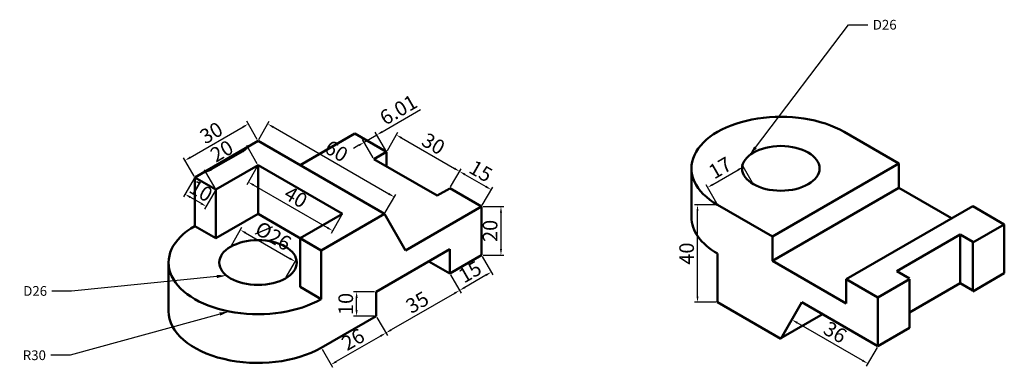
# Model space of a CAD drawing. Units: millimetres. Extents: x 2898 to 3303, y 965 to 1108.
import ezdxf
from ezdxf import colors
from ezdxf.entities.mleader import LeaderData, LeaderLine
from ezdxf.math import Vec2, Vec3

# ---------------------------------------------------------------- set-up
doc = ezdxf.new("R2010")
doc.units = ezdxf.units.MM
doc.layers.add('M-DIMS', color=2, linetype='Continuous', lineweight=25)
doc.layers.add('M-OUTL', color=7, linetype='Continuous', lineweight=50)
doc.styles.get("Standard").update_dxf_attribs({"font": 'arial.ttf'})
doc.dimstyles.new('ISO-25', dxfattribs={"dimtxt": 6, "dimasz": 2.5, "dimexe": 1.25, "dimexo": 0.625, "dimtad": 1, "dimtxsty": 'Standard', "dimcen": 2.5, "dimadec": 0, "dimazin": 0, "dimtfac": 1, "dimtmove": 0, "dimatfit": 3, "dimfxl": 1, "dimarcsym": 0})

# ---------------------------------------------------------------- blocks, each defined once
blk = doc.blocks.new('*D1')
at = {"layer": 'Defpoints', "color": 0, "transparency": 16777216}
for p in [(2992.16, 1065.01), (2996.16, 1058.09), (2970.18, 1043.09)]:
    blk.add_point(p, dxfattribs=at)
at = {"layer": 'M-DIMS', "color": 0, "lineweight": -2, "transparency": 16777216}
for p, q in [((2968.35, 1051.26), (2990, 1063.76)), ((2995.85, 1058.63), (2991.54, 1066.1)), ((2969.87, 1043.63), (2965.56, 1051.1))]:
    blk.add_line(p, q, dxfattribs=at)
at = {"layer": 'M-DIMS', "color": 0, "transparency": 16777216}
for points in [[(2989.79, 1064.12), (2990.21, 1063.4), (2992.16, 1065.01)], [(2968.14, 1051.62), (2968.56, 1050.9), (2966.18, 1050.01)]]:
    blk.add_solid(points, dxfattribs=at)
at = {"layer": 'M-DIMS', "color": 0, "transparency": 16777216, "insert": (2977.33, 1060.71), "char_height": 6, "attachment_point": 5, "rotation": 30}
blk.add_mtext('30', dxfattribs=at)
blk = doc.blocks.new('*D2')
at = {"layer": 'Defpoints', "color": 0, "transparency": 16777216}
for p in [(2992.16, 1055.01), (2996.16, 1048.09), (2978.84, 1038.09)]:
    blk.add_point(p, dxfattribs=at)
at = {"layer": 'M-DIMS', "color": 0, "lineweight": -2, "transparency": 16777216}
for p, q in [((2995.85, 1048.63), (2991.54, 1056.1)), ((2977.01, 1046.26), (2990, 1053.76)), ((2978.53, 1038.63), (2974.22, 1046.1))]:
    blk.add_line(p, q, dxfattribs=at)
at = {"layer": 'M-DIMS', "color": 0, "transparency": 16777216}
for points in [[(2989.79, 1054.12), (2990.21, 1053.4), (2992.16, 1055.01)], [(2976.8, 1046.62), (2977.22, 1045.9), (2974.84, 1045.01)]]:
    blk.add_solid(points, dxfattribs=at)
at = {"layer": 'M-DIMS', "color": 0, "transparency": 16777216, "insert": (2981.66, 1053.21), "char_height": 6, "attachment_point": 5, "rotation": 30}
blk.add_mtext('20', dxfattribs=at)
blk = doc.blocks.new('*D3')
at = {"layer": 'Defpoints', "color": 0, "transparency": 16777216}
for p in [(2996.16, 1048.09), (2992.16, 1041.16), (3030.8, 1028.09)]:
    blk.add_point(p, dxfattribs=at)
at = {"layer": 'M-DIMS', "color": 0, "lineweight": -2, "transparency": 16777216}
for p, q in [((2995.85, 1047.54), (2991.54, 1040.07)), ((3024.64, 1022.41), (2994.33, 1039.91)), ((3030.49, 1027.54), (3026.18, 1020.07))]:
    blk.add_line(p, q, dxfattribs=at)
at = {"layer": 'M-DIMS', "color": 0, "transparency": 16777216}
for points in [[(2994.54, 1040.27), (2994.12, 1039.55), (2992.16, 1041.16)], [(3024.85, 1022.77), (3024.43, 1022.05), (3026.8, 1021.16)]]:
    blk.add_solid(points, dxfattribs=at)
at = {"layer": 'M-DIMS', "color": 0, "transparency": 16777216, "insert": (3011.33, 1034.35), "char_height": 6, "attachment_point": 5, "rotation": 330}
blk.add_mtext('40', dxfattribs=at)
blk = doc.blocks.new('*D4')
at = {"layer": 'Defpoints', "color": 0, "transparency": 16777216}
for p in [(2970.18, 1043.09), (2966.18, 1036.16), (2978.84, 1038.09)]:
    blk.add_point(p, dxfattribs=at)
at = {"layer": 'M-DIMS', "color": 0, "lineweight": -2, "transparency": 16777216}
for p, q in [((2969.87, 1042.54), (2965.56, 1035.07)), ((2978.53, 1037.54), (2974.22, 1030.07)), ((2972.68, 1032.41), (2968.35, 1034.91))]:
    blk.add_line(p, q, dxfattribs=at)
at = {"layer": 'M-DIMS', "color": 0, "transparency": 16777216}
for points in [[(2968.56, 1035.27), (2968.14, 1034.55), (2966.18, 1036.16)], [(2972.89, 1032.77), (2972.47, 1032.05), (2974.84, 1031.16)]]:
    blk.add_solid(points, dxfattribs=at)
at = {"layer": 'M-DIMS', "color": 0, "transparency": 16777216, "insert": (2972.36, 1036.85), "char_height": 6, "attachment_point": 5, "rotation": 330}
blk.add_mtext('10', dxfattribs=at)
blk = doc.blocks.new('*D5')
at = {"layer": 'Defpoints', "color": 0, "transparency": 16777216}
for p in [(3087.96, 1031.09), (3087.96, 1011.09), (3095.96, 1011.09)]:
    blk.add_point(p, dxfattribs=at)
at = {"layer": 'M-DIMS', "color": 0, "lineweight": -2, "transparency": 16777216}
for p, q in [((3088.59, 1031.09), (3097.21, 1031.09)), ((3095.96, 1028.59), (3095.96, 1013.59)), ((3088.59, 1011.09), (3097.21, 1011.09))]:
    blk.add_line(p, q, dxfattribs=at)
at = {"layer": 'M-DIMS', "color": 0, "transparency": 16777216}
for points in [[(3095.55, 1028.59), (3096.38, 1028.59), (3095.96, 1031.09)], [(3095.55, 1013.59), (3096.38, 1013.59), (3095.96, 1011.09)]]:
    blk.add_solid(points, dxfattribs=at)
at = {"layer": 'M-DIMS', "color": 0, "transparency": 16777216, "insert": (3092.27, 1021.09), "char_height": 6, "attachment_point": 5, "rotation": 90}
blk.add_mtext('20', dxfattribs=at)
blk = doc.blocks.new('*D6')
at = {"layer": 'Defpoints', "color": 0, "transparency": 16777216}
for p in [(3044.66, 986.09), (3022.14, 973.09), (3026.14, 966.16)]:
    blk.add_point(p, dxfattribs=at)
at = {"layer": 'M-DIMS', "color": 0, "lineweight": -2, "transparency": 16777216}
for p, q in [((3044.97, 985.54), (3049.29, 978.07)), ((3046.5, 977.91), (3028.31, 967.41)), ((3022.46, 972.54), (3026.77, 965.07))]:
    blk.add_line(p, q, dxfattribs=at)
at = {"layer": 'M-DIMS', "color": 0, "transparency": 16777216}
for points in [[(3046.29, 978.27), (3046.7, 977.55), (3048.66, 979.16)], [(3028.1, 967.77), (3028.52, 967.05), (3026.14, 966.16)]]:
    blk.add_solid(points, dxfattribs=at)
at = {"layer": 'M-DIMS', "color": 0, "transparency": 16777216, "insert": (3035.56, 975.85), "char_height": 6, "attachment_point": 5, "rotation": 30}
blk.add_mtext('26', dxfattribs=at)
blk = doc.blocks.new('*D7')
at = {"layer": 'Defpoints', "color": 0, "transparency": 16777216}
for p in [(3074.97, 1003.59), (3044.66, 986.09), (3048.66, 979.16)]:
    blk.add_point(p, dxfattribs=at)
at = {"layer": 'M-DIMS', "color": 0, "lineweight": -2, "transparency": 16777216}
for p, q in [((3075.28, 1003.04), (3079.6, 995.57)), ((3076.81, 995.41), (3050.83, 980.41)), ((3044.97, 985.54), (3049.29, 978.07))]:
    blk.add_line(p, q, dxfattribs=at)
at = {"layer": 'M-DIMS', "color": 0, "transparency": 16777216}
for points in [[(3076.6, 995.77), (3077.02, 995.05), (3078.97, 996.66)], [(3050.62, 980.77), (3051.03, 980.05), (3048.66, 979.16)]]:
    blk.add_solid(points, dxfattribs=at)
at = {"layer": 'M-DIMS', "color": 0, "transparency": 16777216, "insert": (3061.97, 991.1), "char_height": 6, "attachment_point": 5, "rotation": 30}
blk.add_mtext('35', dxfattribs=at)
blk = doc.blocks.new('*D8')
at = {"layer": 'Defpoints', "color": 0, "transparency": 16777216}
for p in [(3087.96, 1011.09), (3074.97, 1003.59), (3078.97, 996.66)]:
    blk.add_point(p, dxfattribs=at)
at = {"layer": 'M-DIMS', "color": 0, "lineweight": -2, "transparency": 16777216}
for p, q in [((3088.28, 1010.54), (3092.59, 1003.07)), ((3075.28, 1003.04), (3079.6, 995.57)), ((3089.8, 1002.91), (3081.14, 997.91))]:
    blk.add_line(p, q, dxfattribs=at)
at = {"layer": 'M-DIMS', "color": 0, "transparency": 16777216}
for points in [[(3089.59, 1003.27), (3090.01, 1002.55), (3091.96, 1004.16)], [(3080.93, 998.27), (3081.35, 997.55), (3078.97, 996.66)]]:
    blk.add_solid(points, dxfattribs=at)
at = {"layer": 'M-DIMS', "color": 0, "transparency": 16777216, "insert": (3083.62, 1003.6), "char_height": 6, "attachment_point": 5, "rotation": 30}
blk.add_mtext('15', dxfattribs=at)
blk = doc.blocks.new('*D9')
at = {"layer": 'Defpoints', "color": 0, "transparency": 16777216}
for p in [(3036.66, 996.09), (3044.66, 996.09), (3044.66, 986.09)]:
    blk.add_point(p, dxfattribs=at)
at = {"layer": 'M-DIMS', "color": 0, "lineweight": -2, "transparency": 16777216}
for p, q in [((3044.04, 996.09), (3035.41, 996.09)), ((3036.66, 988.59), (3036.66, 993.59)), ((3044.04, 986.09), (3035.41, 986.09))]:
    blk.add_line(p, q, dxfattribs=at)
at = {"layer": 'M-DIMS', "color": 0, "transparency": 16777216}
for points in [[(3036.24, 993.59), (3037.08, 993.59), (3036.66, 996.09)], [(3036.24, 988.59), (3037.08, 988.59), (3036.66, 986.09)]]:
    blk.add_solid(points, dxfattribs=at)
at = {"layer": 'M-DIMS', "color": 0, "transparency": 16777216, "insert": (3032.97, 991.09), "char_height": 6, "attachment_point": 5, "rotation": 90}
blk.add_mtext('10', dxfattribs=at)
blk = doc.blocks.new('*D10')
at = {"layer": 'Defpoints', "color": 0, "transparency": 16777216}
for p in [(3048.99, 1053.59), (3078.97, 1045.51), (3074.97, 1038.59)]:
    blk.add_point(p, dxfattribs=at)
at = {"layer": 'M-DIMS', "color": 0, "lineweight": -2, "transparency": 16777216}
for p, q in [((3049.3, 1054.13), (3053.62, 1061.6)), ((3055.16, 1059.26), (3076.81, 1046.76)), ((3075.28, 1039.13), (3079.6, 1046.6))]:
    blk.add_line(p, q, dxfattribs=at)
at = {"layer": 'M-DIMS', "color": 0, "transparency": 16777216}
for points in [[(3055.36, 1059.62), (3054.95, 1058.9), (3052.99, 1060.51)], [(3077.02, 1047.12), (3076.6, 1046.4), (3078.97, 1045.51)]]:
    blk.add_solid(points, dxfattribs=at)
at = {"layer": 'M-DIMS', "color": 0, "transparency": 16777216, "insert": (3067.83, 1056.21), "char_height": 6, "attachment_point": 5, "rotation": 330}
blk.add_mtext('30', dxfattribs=at)
blk = doc.blocks.new('*D11')
at = {"layer": 'Defpoints', "color": 0, "transparency": 16777216}
for p in [(3074.97, 1038.59), (3091.96, 1038.01), (3087.96, 1031.09)]:
    blk.add_point(p, dxfattribs=at)
at = {"layer": 'M-DIMS', "color": 0, "lineweight": -2, "transparency": 16777216}
for p, q in [((3075.28, 1039.13), (3079.6, 1046.6)), ((3081.14, 1044.26), (3089.8, 1039.26)), ((3088.28, 1031.63), (3092.59, 1039.1))]:
    blk.add_line(p, q, dxfattribs=at)
at = {"layer": 'M-DIMS', "color": 0, "transparency": 16777216}
for points in [[(3081.35, 1044.62), (3080.93, 1043.9), (3078.97, 1045.51)], [(3090.01, 1039.62), (3089.59, 1038.9), (3091.96, 1038.01)]]:
    blk.add_solid(points, dxfattribs=at)
at = {"layer": 'M-DIMS', "color": 0, "transparency": 16777216, "insert": (3087.31, 1044.96), "char_height": 6, "attachment_point": 5, "rotation": 330}
blk.add_mtext('15', dxfattribs=at)
blk = doc.blocks.new('*D12')
at = {"layer": 'Defpoints', "color": 0, "transparency": 16777216}
for p in [(2996.16, 1058.09), (3052.13, 1035.01), (3048.13, 1028.09)]:
    blk.add_point(p, dxfattribs=at)
at = {"layer": 'M-DIMS', "color": 0, "lineweight": -2, "transparency": 16777216}
for p, q in [((2996.48, 1058.63), (3000.79, 1066.1)), ((3002.33, 1063.76), (3049.96, 1036.26)), ((3048.44, 1028.63), (3052.75, 1036.1))]:
    blk.add_line(p, q, dxfattribs=at)
at = {"layer": 'M-DIMS', "color": 0, "transparency": 16777216}
for points in [[(3002.54, 1064.12), (3002.12, 1063.4), (3000.16, 1065.01)], [(3050.17, 1036.62), (3049.75, 1035.9), (3052.13, 1035.01)]]:
    blk.add_solid(points, dxfattribs=at)
at = {"layer": 'M-DIMS', "color": 0, "transparency": 16777216, "insert": (3027.99, 1053.21), "char_height": 6, "attachment_point": 5, "rotation": 330}
blk.add_mtext('60', dxfattribs=at)
blk = doc.blocks.new('*D13')
at = {"layer": 'Defpoints', "color": 0, "transparency": 16777216}
for p in [(3176.7, 1031.76), (3184.95, 1031.76), (3184.95, 991.76)]:
    blk.add_point(p, dxfattribs=at)
at = {"layer": 'M-DIMS', "color": 0, "lineweight": -2, "transparency": 16777216}
for p, q in [((3184.33, 1031.76), (3175.45, 1031.76)), ((3176.7, 994.26), (3176.7, 1029.26)), ((3184.33, 991.76), (3175.45, 991.76))]:
    blk.add_line(p, q, dxfattribs=at)
at = {"layer": 'M-DIMS', "color": 0, "transparency": 16777216}
for points in [[(3176.29, 1029.26), (3177.12, 1029.26), (3176.7, 1031.76)], [(3176.29, 994.26), (3177.12, 994.26), (3176.7, 991.76)]]:
    blk.add_solid(points, dxfattribs=at)
at = {"layer": 'M-DIMS', "color": 0, "transparency": 16777216, "insert": (3173.02, 1011.76), "char_height": 6, "attachment_point": 5, "rotation": 90}
blk.add_mtext('40', dxfattribs=at)
blk = doc.blocks.new('*D14')
at = {"layer": 'Defpoints', "color": 0, "transparency": 16777216}
for p in [(3219.59, 991.76), (3215.47, 984.62), (3250.77, 973.76)]:
    blk.add_point(p, dxfattribs=at)
at = {"layer": 'M-DIMS', "color": 0, "lineweight": -2, "transparency": 16777216}
for p, q in [((3219.28, 991.22), (3214.84, 983.53)), ((3244.48, 967.87), (3217.63, 983.37)), ((3250.46, 973.22), (3246.02, 965.53))]:
    blk.add_line(p, q, dxfattribs=at)
at = {"layer": 'M-DIMS', "color": 0, "transparency": 16777216}
for points in [[(3217.84, 983.73), (3217.43, 983.01), (3215.47, 984.62)], [(3244.69, 968.23), (3244.27, 967.51), (3246.65, 966.62)]]:
    blk.add_solid(points, dxfattribs=at)
at = {"layer": 'M-DIMS', "color": 0, "transparency": 16777216, "insert": (3232.9, 978.81), "char_height": 6, "attachment_point": 5, "rotation": 330}
blk.add_mtext('36', dxfattribs=at)
blk = doc.blocks.new('*D15')
at = {"layer": 'Defpoints', "color": 0, "transparency": 16777216}
for p in [(2984.91, 1014.59), (3011.42, 1008.51), (3007.42, 1001.59)]:
    blk.add_point(p, dxfattribs=at)
at = {"layer": 'M-DIMS', "color": 0, "lineweight": -2, "transparency": 16777216}
for p, q in [((2985.22, 1015.13), (2989.53, 1022.6)), ((2991.07, 1020.26), (3009.26, 1009.76)), ((3007.73, 1002.13), (3012.05, 1009.6))]:
    blk.add_line(p, q, dxfattribs=at)
at = {"layer": 'M-DIMS', "color": 0, "transparency": 16777216}
for points in [[(2991.28, 1020.62), (2990.86, 1019.9), (2988.91, 1021.51)], [(3009.47, 1010.12), (3009.05, 1009.4), (3011.42, 1008.51)]]:
    blk.add_solid(points, dxfattribs=at)
at = {"layer": 'M-DIMS', "color": 0, "transparency": 16777216, "insert": (3002.09, 1018.35), "char_height": 6, "attachment_point": 5, "rotation": 330}
blk.add_mtext('%%c26', dxfattribs=at)
blk = doc.blocks.new('*D16')
at = {"layer": 'Defpoints', "color": 0, "transparency": 16777216}
for p in [(3195.55, 1047.41), (3199.68, 1040.26), (3184.95, 1031.76)]:
    blk.add_point(p, dxfattribs=at)
at = {"layer": 'M-DIMS', "color": 0, "lineweight": -2, "transparency": 16777216}
for p, q in [((3199.36, 1040.8), (3194.93, 1048.49)), ((3182.99, 1040.16), (3193.39, 1046.16)), ((3184.64, 1032.3), (3180.2, 1039.99))]:
    blk.add_line(p, q, dxfattribs=at)
at = {"layer": 'M-DIMS', "color": 0, "transparency": 16777216}
for points in [[(3193.18, 1046.52), (3193.59, 1045.8), (3195.55, 1047.41)], [(3182.79, 1040.52), (3183.2, 1039.8), (3180.83, 1038.91)]]:
    blk.add_solid(points, dxfattribs=at)
at = {"layer": 'M-DIMS', "color": 0, "transparency": 16777216, "insert": (3186.37, 1046.31), "char_height": 6, "attachment_point": 5, "rotation": 30}
blk.add_mtext('17', dxfattribs=at)
blk = doc.blocks.new('*D17')
at = {"layer": 'Defpoints', "color": 0, "transparency": 16777216}
for p in [(3044.97, 1060.5), (3048.99, 1053.59), (3043.8, 1050.57)]:
    blk.add_point(p, dxfattribs=at)
at = {"layer": 'M-DIMS', "color": 0, "lineweight": -2, "transparency": 16777216}
for p, q in [((3047.13, 1061.76), (3062.88, 1070.91)), ((3039.78, 1057.48), (3044.97, 1060.5)), ((3048.68, 1054.13), (3044.34, 1061.58)), ((3037.61, 1056.23), (3035.45, 1054.97)), ((3043.48, 1051.11), (3039.15, 1058.56))]:
    blk.add_line(p, q, dxfattribs=at)
at = {"layer": 'M-DIMS', "color": 0, "transparency": 16777216}
for points in [[(3046.92, 1062.12), (3047.34, 1061.4), (3044.97, 1060.5)], [(3037.41, 1056.59), (3037.82, 1055.87), (3039.78, 1057.48)]]:
    blk.add_solid(points, dxfattribs=at)
at = {"layer": 'M-DIMS', "color": 0, "transparency": 16777216, "insert": (3054.23, 1070.15), "char_height": 6, "attachment_point": 5, "rotation": 30.1591}
blk.add_mtext('6.01', dxfattribs=at)

msp = doc.modelspace()

# ---------------------------------------------------------------- linework, layer by layer
at = {"layer": 'M-OUTL'}
for p, q in [((3036.001, 1061.085), (3013.484, 1048.085)), ((3036.001, 1061.085), (3013.484, 1048.085)), ((3048.991, 1053.585), (3036.001, 1061.085)), ((3259.432, 1048.762), (3236.915, 1061.762)), ((2970.183, 1043.085), (2996.164, 1058.085)), ((2996.164, 1058.085), (3048.125, 1028.085)), ((3043.795, 1050.566), (3048.991, 1053.566)), ((3048.991, 1047.566), (3048.991, 1053.566)), ((2978.843, 1038.085), (2996.164, 1048.085)), ((2996.164, 1048.085), (3030.805, 1028.085)), ((2996.164, 1028.085), (2996.164, 1048.085)), ((3069.776, 1035.566), (3043.795, 1050.566)), ((3207.471, 1018.762), (3259.432, 1048.762)), ((3259.432, 1048.762), (3259.432, 1038.762)), ((3174.192, 1046.762), (3174.192, 1026.762)), ((2970.183, 1023.085), (2970.183, 1043.085)), ((2978.843, 1038.066), (2970.183, 1043.066)), ((2978.843, 1018.085), (2978.843, 1038.085)), ((3069.776, 1035.566), (3074.972, 1038.566)), ((3087.963, 1031.085), (3074.972, 1038.585)), ((3207.471, 1008.762), (3259.432, 1038.762)), ((3259.432, 1038.762), (3281.083, 1026.262)), ((3184.954, 1031.762), (3207.471, 1018.762)), ((2978.843, 1018.085), (2996.164, 1028.085)), ((2996.164, 1028.085), (3022.145, 1013.085)), ((3030.805, 1028.085), (3013.484, 1018.085)), ((3048.125, 1028.085), (3022.145, 1013.085)), ((3056.786, 1013.085), (3048.125, 1028.085)), ((3056.786, 1013.085), (3087.963, 1031.085)), ((3087.963, 1011.085), (3087.963, 1031.085)), ((3237.781, 1001.262), (3289.743, 1031.262)), ((3289.743, 1031.262), (3302.733, 1023.762)), ((3302.733, 1023.762), (3289.743, 1031.262)), ((3289.743, 1016.262), (3302.733, 1023.762)), ((3302.733, 1023.762), (3302.733, 1003.762)), ((2970.183, 1023.085), (2978.843, 1018.085)), ((3258.57, 1004.566), (3284.55, 1019.566)), ((3289.746, 1016.566), (3284.55, 1019.566)), ((3284.55, 999.566), (3284.55, 1019.566)), ((3013.484, 1018.085), (3022.145, 1013.085)), ((3013.484, 998.085), (3013.484, 1018.085)), ((3207.471, 1008.762), (3207.471, 1018.762)), ((3289.743, 996.262), (3289.743, 1016.262)), ((3022.145, 1013.085), (3022.145, 993.085)), ((3074.972, 1013.585), (3044.661, 996.085)), ((3074.972, 1003.585), (3074.972, 1013.585)), ((3184.954, 1011.762), (3184.954, 991.762)), ((2959.422, 1008.085), (2959.422, 988.085)), ((3074.972, 1003.566), (3066.312, 1008.566)), ((3087.963, 1011.085), (3074.972, 1003.585)), ((3237.781, 991.262), (3207.471, 1008.762)), ((3263.766, 1001.566), (3258.57, 1004.566)), ((3302.733, 1003.762), (3289.743, 996.262)), ((3250.772, 993.762), (3237.781, 1001.262)), ((3237.781, 1001.262), (3237.781, 991.262)), ((3263.762, 1001.262), (3250.772, 993.762)), ((3263.762, 981.262), (3263.762, 1001.262)), ((3263.766, 987.566), (3284.55, 999.566)), ((3289.746, 996.566), (3284.55, 999.566)), ((3022.145, 993.085), (3013.484, 998.085)), ((3044.661, 996.085), (3044.661, 986.085)), ((3184.954, 991.762), (3210.935, 976.762)), ((3210.935, 976.762), (3219.595, 991.762)), ((3250.772, 973.762), (3219.595, 991.762)), ((3250.772, 973.762), (3250.772, 993.762)), ((3210.938, 977.066), (3228.259, 987.066)), ((3044.661, 986.085), (3022.145, 973.085)), ((3250.772, 973.762), (3263.762, 981.262))]:
    msp.add_line(p, q, dxfattribs=at)
for centre, start_param, end_param in [((3210.935, 1046.762), 3.9269908, 7.0685835), ((3210.935, 1026.762), 6.2831853, 7.0685835), ((2996.164, 1008.085), 5.4977871, 8.6393798), ((2996.164, 988.085), 6.2831853, 8.6393798)]:
    msp.add_ellipse(centre, major_axis=(-36.742, 0), ratio=0.5773503, start_param=start_param, end_param=end_param, dxfattribs=at)
for centre in [(3210.935, 1046.762), (2996.164, 1008.085)]:
    msp.add_ellipse(centre, major_axis=(-15.922, 0), ratio=0.5773503, dxfattribs=at)

# ---------------------------------------------------------------- dimensions: what is measured, and where the dimension line sits
at = {"layer": 'M-DIMS'}
for base, p1, p2, angle, override, picture, middle in [((3044.972, 1060.502), (3043.795, 1050.566), (3048.991, 1053.585), 30.15914, {"dimdec": 2, "dimlfac": 1, "dimrnd": 0, "dimzin": 0, "dimdsep": 46, "dimlunit": 2}, '*D17', (3054.234, 1070.15)), ((2992.164, 1065.013), (2970.183, 1043.085), (2996.164, 1058.085), 30, {"dimdec": 0, "dimlfac": 1, "dimrnd": 0, "dimzin": 0, "dimdsep": 46, "dimlunit": 2}, '*D1', (2977.328, 1060.709)), ((3052.125, 1035.013), (2996.164, 1058.085), (3048.125, 1028.085), 330, {"dimdec": 0, "dimlfac": 1, "dimrnd": 0, "dimzin": 0, "dimdsep": 46, "dimlunit": 2}, '*D12', (3027.989, 1053.208)), ((3078.972, 1045.513), (3048.991, 1053.585), (3074.972, 1038.585), 330, {"dimdec": 0, "dimlfac": 1, "dimrnd": 0, "dimzin": 0, "dimdsep": 46, "dimlunit": 2}, '*D10', (3067.827, 1056.209)), ((2992.164, 1055.013), (2978.843, 1038.085), (2996.164, 1048.085), 30, {"dimdec": 0, "dimlfac": 1, "dimrnd": 0, "dimzin": 0, "dimdsep": 46, "dimlunit": 2}, '*D2', (2981.659, 1053.208)), ((3195.551, 1047.407), (3184.954, 1031.762), (3199.676, 1040.262), 30, {"dimdec": 0, "dimlfac": 1, "dimrnd": 0, "dimzin": 0, "dimdsep": 46, "dimlunit": 2}, '*D16', (3186.371, 1046.307)), ((2992.164, 1041.157), (3030.805, 1028.085), (2996.164, 1048.085), 150, {"dimdec": 0, "dimlfac": 1, "dimrnd": 0, "dimzin": 0, "dimdsep": 46, "dimlunit": 2}, '*D3', (3011.329, 1034.351)), ((3091.963, 1038.013), (3074.972, 1038.585), (3087.963, 1031.085), 330, {"dimdec": 0, "dimlfac": 1, "dimrnd": 0, "dimzin": 0, "dimdsep": 46, "dimlunit": 2}, '*D11', (3087.312, 1044.958)), ((2966.183, 1036.157), (2978.843, 1038.085), (2970.183, 1043.085), 150, {"dimdec": 0, "dimlfac": 1, "dimrnd": 0, "dimzin": 0, "dimdsep": 46, "dimlunit": 2}, '*D4', (2972.357, 1036.851)), ((3176.704, 1031.762), (3184.954, 991.762), (3184.954, 1031.762), 90, {"dimdec": 0, "dimlfac": 1, "dimrnd": 0, "dimzin": 0, "dimdsep": 46, "dimlunit": 2}, '*D13', (3173.015, 1011.762)), ((3095.963, 1011.085), (3087.963, 1031.085), (3087.963, 1011.085), 270, {"dimdec": 0, "dimlfac": 1, "dimrnd": 0, "dimzin": 0, "dimdsep": 46, "dimlunit": 2}, '*D5', (3092.274, 1021.085)), ((3078.972, 996.657), (3087.963, 1011.085), (3074.972, 1003.585), 210, {"dimdec": 0, "dimlfac": 1, "dimrnd": 0, "dimzin": 0, "dimdsep": 46, "dimlunit": 2}, '*D8', (3083.623, 1003.601)), ((3048.661, 979.157), (3074.972, 1003.585), (3044.661, 986.085), 210, {"dimdec": 0, "dimlfac": 1, "dimrnd": 0, "dimzin": 0, "dimdsep": 46, "dimlunit": 2}, '*D7', (3061.971, 991.103)), ((3036.661, 996.085), (3044.661, 986.085), (3044.661, 996.085), 90, {"dimdec": 0, "dimlfac": 1, "dimrnd": 0, "dimzin": 0, "dimdsep": 46, "dimlunit": 2}, '*D9', (3032.973, 991.085)), ((3215.47, 984.617), (3250.772, 973.762), (3219.595, 991.762), 150, {"dimdec": 0, "dimlfac": 1, "dimrnd": 0, "dimzin": 0, "dimdsep": 46, "dimlunit": 2}, '*D14', (3232.904, 978.813)), ((3026.145, 966.157), (3044.661, 986.085), (3022.145, 973.085), 210, {"dimdec": 0, "dimlfac": 1, "dimrnd": 0, "dimzin": 0, "dimdsep": 46, "dimlunit": 2}, '*D6', (3035.559, 975.851))]:
    dim = msp.add_linear_dim(base=base, p1=p1, p2=p2, angle=angle, dimstyle='ISO-25', override=override, dxfattribs=at)
    dim.commit()
    dim.dimension.update_dxf_attribs({"geometry": picture, "text_midpoint": middle})
dim = msp.add_linear_dim(base=(3011.422, 1008.513), p1=(2984.906, 1014.585), p2=(3007.422, 1001.585), angle=330, text='%%c<>', dimstyle='ISO-25', override={"dimdec": 0, "dimlfac": 1, "dimrnd": 0, "dimzin": 0, "dimdsep": 46, "dimlunit": 2}, dxfattribs=at)
dim.commit()
dim.dimension.update_dxf_attribs({"geometry": '*D15', "text_midpoint": (3002.092, 1018.353)})

# ---------------------------------------------------------------- leaders
ml = msp.add_multileader_mtext('Standard', dxfattribs=at)
ml.set_content('D26', color=256)
ml.set_leader_properties()
ml.build(insert=Vec2(0, 0))
ctx = ml.context
ctx.base_point, ctx.plane_origin = Vec3(3246.701, 1105.714), Vec3(3198.054, 1052.166)
notes = []
notes.append((ctx, [(0, (1, 1, 0), (3238.701, 1105.714), (1, 0), 8, [(0, [(3198.054, 1052.166)], 0, [])])]))
ctx.mtext.insert, ctx.mtext.flow_direction = Vec3(3248.701, 1107.749), 5
ml = msp.add_multileader_mtext('Standard', dxfattribs=at)
ml.set_content('D26', color=256)
ml.set_leader_properties()
ml.build(insert=Vec2(0, 0))
ctx = ml.context
ctx.base_point, ctx.plane_origin = Vec3(2897.957, 996.394), Vec3(2983.188, 1002.758)
ctx.text_align_type = 2
notes.append((ctx, [(0, (1, 1, 0), (2919.52, 996.394), (-1, 0), 8, [(0, [(2983.188, 1002.758)], 0, [])])]))
ctx.mtext.insert, ctx.mtext.alignment, ctx.mtext.flow_direction = Vec3(2909.52, 998.428), 3, 5
ml = msp.add_multileader_mtext('Standard', dxfattribs=at)
ml.set_content('R30', color=256)
ml.set_leader_properties()
ml.build(insert=Vec2(0, 0))
ctx = ml.context
ctx.base_point, ctx.plane_origin = Vec3(2897.512, 969.994), Vec3(2984.306, 988.007)
ctx.text_align_type = 2
notes.append((ctx, [(0, (1, 1, 0), (2919.057, 969.994), (-1, 0), 8, [(0, [(2984.306, 988.007)], 0, [])])]))
ctx.mtext.insert, ctx.mtext.alignment, ctx.mtext.flow_direction = Vec3(2909.057, 972.03), 3, 5
for ctx, leaders in notes:
    for number, flags, end, landing, length, lines in leaders:
        leader = LeaderData()
        leader.index, (leader.has_last_leader_line, leader.has_dogleg_vector, leader.attachment_direction) = number, flags
        leader.last_leader_point, leader.dogleg_vector, leader.dogleg_length = Vec3(end), Vec3(landing), length
        for number, points, colour, breaks in lines:
            line = LeaderLine()
            line.index, line.vertices, line.color, line.breaks = number, Vec3.list(points), colors.encode_raw_color(colour), breaks
            leader.lines.append(line)
        ctx.leaders.append(leader)

doc.saveas('drawing.dxf')
